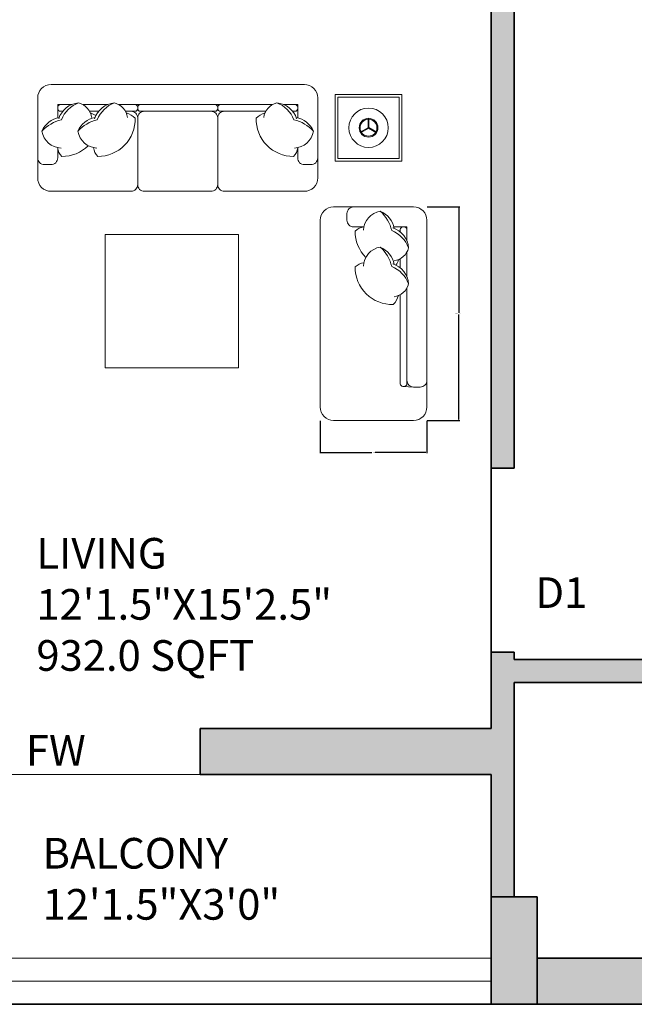
# Model space of a CAD drawing. Units: inches. Extents: x -9 to 505, y -680 to 48.
# Tile 4 of 17: x 235 to 356, y -680 to -487. Entities that reach past the tile are written whole.
import ezdxf

# ---------------------------------------------------------------- set-up
doc = ezdxf.new("R2010")
doc.units = ezdxf.units.IN
doc.header["$MEASUREMENT"] = 0
for name, color, linetype, lineweight in [('A-ANNO-DIMS', 2, 'Continuous', 18), ('A-ANNO-TEXT', 7, 'Continuous', 18), ('A-AREA-IDEN', 7, 'Continuous', 18), ('A-FLOR-HRAL', 4, 'Continuous', 18), ('A-FURN', 8, 'Continuous', 18), ('A-GLAZ', 4, 'Continuous', 18), ('A-WALL', 7, 'Continuous', 35), ('A-WALL-PATT', 251, 'Continuous', 13), ('S-CONC', 7, 'Continuous', 35), ('S-CONC-PATT', 18, 'Continuous', 13)]:
    doc.layers.add(name, color=color, linetype=linetype, lineweight=lineweight)
doc.styles.get("Standard").update_dxf_attribs({"font": 'arial.ttf'})
doc.dimstyles.get("Standard").update_dxf_attribs({"dimtxt": 0.18, "dimasz": 0.18, "dimexe": 0.18, "dimexo": 0.0625, "dimgap": 0.09, "dimtad": 0, "dimtih": 1, "dimtoh": 1, "dimdec": 0, "dimzin": 0, "dimdsep": 46, "dimlunit": 3, "dimtxsty": 'Standard', "dimcen": 0.09, "dimadec": 0, "dimazin": 0, "dimtfac": 1, "dimtdec": 0, "dimtofl": 0, "dimtmove": 0, "dimatfit": 3, "dimfxl": 1, "dimtolj": 1, "dimtzin": 0, "dimarcsym": 0})

# ---------------------------------------------------------------- blocks, each defined once
blk = doc.blocks.new('DAY BED1')
at = {"color": 0}
blk.add_line((0.3, 0.25), (0.225, 0.2549), dxfattribs=at)
blk.add_lwpolyline([(-0.3, 0, -0.414214), (-0.4, 0.1), (-0.4, 0.1, 0.317837), (-0.4, 0.1, -0.414214), (-0.4, 0.1), (-0.4, 0.1, 1.186185), (-0.4, 0.1, -0.414214), (-0.4, 0.1), (-0.4, 1.5, -0.414214), (-0.3, 1.6), (0.3, 1.6, -0.414214), (0.4, 1.5), (0.4, 0.1, -0.414214), (0.3, 0)], format="xyb", close=True, dxfattribs=at)
for points in [[(-0.0725, 1.45), (-0.15, 1.45, -0.414214), (-0.2, 1.5), (-0.2, 1.55, -0.414214), (-0.15, 1.6)], [(-0.0756, 1.4249, -0.356772), (0.0505, 1.5682, -0.249542), (0.1543, 1.4384, 9.61688)], [(0.0505, 1.5682, -0.14773), (0.1364, 1.422, -0.213343), (0.2624, 1.2931, -0.178662)], [(-0.0725, 1.4501, 0.165541), (-0.1386, 1.4192, 0.200231), (-0.0581, 1.2207, 0.121523)], [(0.1433, 1.4422, -0.306663), (0.2624, 1.2931, -0.30633), (0.1536, 1.1957, 0.872847)], [(0.25, 1.3448), (0.25, 1.45), (0.1517, 1.45, -0.414214)], [(0.2, 1.4118), (0.2, 1.43, -0.414214), (0.22, 1.45), (0.23, 1.45, -0.414214), (0.25, 1.43)], [(0.25, 1.43), (0.25, 1.3448, -0.414214)], [(-0.0756, 1.1556, -0.356772), (0.0505, 1.2988, -0.249542), (0.1543, 1.169, 9.61688)], [(0.0505, 1.2988, -0.14773), (0.1364, 1.1527, -0.213343), (0.2624, 1.0238, -0.178662)], [(0.25, 1.2616), (0.25, 1.0755, -0.414214)], [(-0.0725, 1.1808, 0.165541), (-0.1386, 1.1498, 0.425989), (0.1479, 0.869, 0.121523), (0.1873, 0.9357, -7.115464)], [(0.1678, 1.1631, 0.071865), (0.1873, 1.205, -7.115464)], [(0.2, 1.1425), (0.2, 1.2113, -0.414214)], [(0.1433, 1.1729, -0.306663), (0.2624, 1.0238, -0.30633), (0.1536, 0.9263, 0.872847)], [(0.25, 0.9923), (0.25, 0.2749, -0.414214), (0.23, 0.2549), (0.22, 0.2549, -0.414214), (0.2, 0.2749), (0.2, 0.9419, -0.414214)], [(0.25, 0.3775), (0.25, 0.3, 0.414214), (0.3, 0.25), (0.35, 0.25, 0.414214), (0.4, 0.3)]]:
    blk.add_lwpolyline(points, format="xyb", dxfattribs=at)
for points in [[(0.25, 1.0755), (0.25, 1.2616)], [(0.25, 0.3775), (0.25, 0.9923)]]:
    blk.add_lwpolyline(points, dxfattribs=at)
blk = doc.blocks.new('TABLE-COFFEE-SQUARE')
at = {"ltscale": 0.03}
blk.add_lwpolyline([(0, 0), (26.11, 0), (26.11, 26.11), (0, 26.11)], close=True, dxfattribs=at)
blk = doc.blocks.new('*D44')
at = {"layer": 'A-ANNO-DIMS', "color": 0, "lineweight": -2, "transparency": 16777216}
for p, q in [((315.22, -523.45), (321.6, -523.45)), ((321.42, -523.63), (321.42, -544.16)), ((321.42, -565.05), (321.42, -544.52)), ((315.22, -565.23), (321.6, -565.23))]:
    blk.add_line(p, q, dxfattribs=at)
at = {"layer": 'A-ANNO-DIMS', "color": 0, "transparency": 16777216}
for points in [[(321.39, -523.63), (321.45, -523.63), (321.42, -523.45)], [(321.39, -565.05), (321.45, -565.05), (321.42, -565.23)]]:
    blk.add_solid(points, dxfattribs=at)
at = {"layer": 'Defpoints', "color": 0, "transparency": 16777216}
for p in [(315.15, -523.45), (321.42, -523.45), (315.15, -565.23)]:
    blk.add_point(p, dxfattribs=at)
at = {"layer": 'A-ANNO-DIMS', "color": 0, "transparency": 16777216, "insert": (321.42, -544.34), "char_height": 0.18, "attachment_point": 5}
blk.add_mtext('\\A1;DAYBED 3\'-6"', dxfattribs=at)
blk = doc.blocks.new('*D45')
at = {"layer": 'A-ANNO-DIMS', "color": 0, "lineweight": -2, "transparency": 16777216}
for p, q in [((294.27, -565.29), (294.27, -571.67)), ((315.15, -565.29), (315.15, -571.67)), ((294.45, -571.49), (304.39, -571.49)), ((314.97, -571.49), (305.03, -571.49))]:
    blk.add_line(p, q, dxfattribs=at)
at = {"layer": 'A-ANNO-DIMS', "color": 0, "transparency": 16777216}
for points in [[(294.45, -571.46), (294.45, -571.52), (294.27, -571.49)], [(314.97, -571.46), (314.97, -571.52), (315.15, -571.49)]]:
    blk.add_solid(points, dxfattribs=at)
at = {"layer": 'Defpoints', "color": 0, "transparency": 16777216}
for p in [(294.27, -565.23), (315.15, -565.23), (315.15, -571.49)]:
    blk.add_point(p, dxfattribs=at)
at = {"layer": 'A-ANNO-DIMS', "color": 0, "transparency": 16777216, "insert": (304.71, -571.49), "char_height": 0.18, "attachment_point": 5}
blk.add_mtext('\\A1;1\'-9"', dxfattribs=at)

msp = doc.modelspace()

# ---------------------------------------------------------------- hatches: boundary and pattern name
at = {"layer": 'A-WALL-PATT'}
h = msp.add_hatch(color=256, dxfattribs=at)
h.dxf.hatch_style = 1
h.paths.add_polyline_path([(101.64, 11.5), (48.26, 11.5), (48.26, 2.5), (72.26, 2.5), (72.26, -21.25), (81.26, -21.25), (81.26, 2.5), (101.64, 2.5)])
h.paths.add_polyline_path([(36.26, 2.5), (27.26, 2.5), (27.26, -6.92), (36.26, -6.92)])
h.paths.add_polyline_path([(81.26, -57.25), (72.26, -57.25), (72.26, -75.5), (81.26, -75.5)])
h.paths.add_polyline_path([(162.76, 11.5), (137.64, 11.5), (137.64, 2.5), (162.76, 2.5)])
h.paths.add_polyline_path([(179.26, 2.5), (174.76, 2.5), (174.76, -75.5), (179.26, -75.5), (179.26, -54.5), (229.51, -54.5), (229.51, -45.5), (179.26, -45.5)])
h.paths.add_polyline_path([(382.26, -45.5), (332.26, -45.5), (332.26, 2.5), (327.76, 2.5), (327.76, -45.5), (277.51, -45.5), (277.51, -54.5), (327.76, -54.5), (327.76, -111.5), (332.26, -111.5), (332.26, -54.5), (382.26, -54.5)])
h.paths.add_polyline_path([(332.26, -128), (327.76, -128), (327.76, -207), (332.26, -207)])
h.paths.add_polyline_path([(124.76, -111.5), (36.26, -111.5), (36.26, -116), (120.26, -116), (120.26, -168.5), (179.26, -168.5), (179.26, -164), (124.76, -164)])
h.paths.add_polyline_path([(96.26, -164), (36.26, -164), (36.26, -152), (27.26, -152), (27.26, -208.88), (36.26, -208.88), (36.26, -168.5), (96.26, -168.5)])
h.paths.add_polyline_path([(36.26, -244.88), (27.26, -244.88), (27.26, -287), (36.26, -287)])
h.paths.add_polyline_path([(179.26, -204.5), (174.76, -204.5), (174.76, -287), (179.26, -287)])
h.paths.add_polyline_path([(257.26, -296), (248.26, -296), (248.26, -446), (269.26, -446), (269.26, -437), (257.26, -437)])
h.paths.add_polyline_path([(90.26, -296), (81.26, -296), (81.26, -348.67), (90.26, -348.67)])
h.paths.add_polyline_path([(90.26, -384.67), (81.26, -384.67), (81.26, -416), (90.26, -416)])
h.paths.add_polyline_path([(170.26, -452), (36.26, -452), (36.26, -456.5), (165.76, -456.5), (165.76, -504.5), (165.13, -504.5), (165.13, -509), (170.26, -509)])
h.paths.add_polyline_path([(141.76, -504.5), (36.26, -504.5), (36.26, -492.5), (27.26, -492.5), (27.26, -565.96), (36.26, -565.96), (36.26, -509), (141.76, -509)])
h.paths.add_polyline_path([(36.26, -601.96), (27.26, -601.96), (27.26, -658.5), (36.26, -658.5)])
h.paths.add_polyline_path([(170.26, -670.5), (170.26, -634.5), (222.76, -634.5), (222.76, -625.5), (165.76, -625.5), (165.76, -670.5), (36.26, -670.5), (36.26, -679.5), (170.26, -679.5)])
h.paths.add_polyline_path([(332.26, -616.5), (433.89, -616.5), (433.89, -612), (332.26, -612), (332.26, -610.56), (327.76, -610.56), (327.76, -625.5), (270.76, -625.5), (270.76, -634.5), (327.76, -634.5), (327.76, -658.5), (332.26, -658.5)])
h.paths.add_polyline_path([(459.76, -670.5), (336.76, -670.5), (336.76, -679.5), (459.76, -679.5)])
h.paths.add_polyline_path([(468.76, -545.74), (459.76, -545.74), (459.76, -612), (457.89, -612), (457.89, -616.5), (459.76, -616.5), (459.76, -658.5), (468.76, -658.5)])
h.paths.add_polyline_path([(332.26, -446), (327.76, -446), (327.76, -574.56), (332.26, -574.56)])
h.paths.add_polyline_path([(327.76, -437), (305.26, -437), (305.26, -446), (327.76, -446)])
h.paths.add_polyline_path([(459.76, -437), (348.76, -437), (348.76, -446), (459.76, -446)])
h.paths.add_polyline_path([(468.76, -458), (459.76, -458), (459.76, -509.74), (468.76, -509.74)])
h.paths.add_polyline_path([(468.76, -365), (459.76, -365), (459.76, -437), (468.76, -437)])
h.paths.add_polyline_path([(468.76, -299.6), (459.76, -299.6), (459.76, -344), (468.76, -344)])
h.paths.add_polyline_path([(468.76, -184.74), (459.76, -184.74), (459.76, -231), (401.26, -231), (401.26, -235.5), (459.76, -235.5), (459.76, -275.6), (468.76, -275.6)])
h.paths.add_polyline_path([(390.76, -356), (342.76, -356), (342.76, -365), (390.76, -365)])
h.paths.add_polyline_path([(459.76, -356), (405.76, -356), (405.76, -365), (459.76, -365)])
h.paths.add_polyline_path([(405.76, -296), (396.76, -296), (396.76, -356), (405.76, -356)])
h.paths.add_polyline_path([(336.76, -296), (327.76, -296), (327.76, -356), (336.76, -356)])
h.paths.add_polyline_path([(468.76, -9.5), (459.76, -9.5), (459.76, -45.5), (418.26, -45.5), (418.26, -54.5), (468.76, -54.5)])
h.paths.add_polyline_path([(468.76, -54.5), (459.76, -54.5), (459.76, -111.5), (468.76, -111.5)])
h.paths.add_polyline_path([(468.76, -128), (459.76, -128), (459.76, -148.74), (468.76, -148.74)])
at = {"layer": 'S-CONC-PATT'}
h = msp.add_hatch(color=256, dxfattribs=at)
h.dxf.hatch_style = 1
h.paths.add_polyline_path([(336.76, -658.5), (327.76, -658.5), (327.76, -679.5), (336.76, -679.5), (336.76, -670.5)])
h.paths.add_polyline_path([(468.76, -658.5), (459.76, -658.5), (459.76, -679.5), (468.76, -679.5)])
h.paths.add_polyline_path([(36.26, -658.5), (27.26, -658.5), (27.26, -679.5), (36.26, -679.5)])

# ---------------------------------------------------------------- linework, layer by layer
at = {"layer": 'A-FLOR-HRAL'}
for p, q in [((327.76, -670.5), (170.26, -670.5)), ((170.26, -670.5), (327.76, -670.5)), ((327.76, -679.5), (327.76, -670.5)), ((170.26, -675), (327.76, -675)), ((170.26, -679.5), (327.76, -679.5))]:
    msp.add_line(p, q, dxfattribs=at)
at = {"layer": 'A-FURN'}
for p, q in [((303.64, -507.96), (303.64, -506.12)), ((303.81, -507.96), (303.81, -506.12)), ((303.69, -507.89), (302.09, -508.81)), ((303.77, -508.03), (302.17, -508.95)), ((303.69, -508.03), (305.28, -508.95)), ((303.77, -507.89), (305.36, -508.81))]:
    msp.add_line(p, q, dxfattribs=at)
at = {"layer": 'A-FURN', "ltscale": 0.03}
msp.add_lwpolyline([(293.77, -517.79, -0.414214), (291.16, -520.4), (275.49, -520.4, -0.414214), (274.19, -519.09, -0.414214), (272.88, -520.4), (259.83, -520.4, -0.414214), (258.52, -519.09, -0.414214), (257.22, -520.4), (241.55, -520.4, -0.414214), (238.94, -517.79), (238.94, -502.12, -0.414214), (241.55, -499.51), (291.16, -499.51, -0.414214), (293.77, -502.12)], format="xyb", close=True, dxfattribs=at)
msp.add_lwpolyline([(310.25, -514.49), (297.2, -514.49), (297.2, -501.43), (310.25, -501.43)], close=True, dxfattribs=at)
at = {"layer": 'A-FURN'}
msp.add_lwpolyline([(297.72, -513.97), (309.73, -513.97), (309.73, -501.96), (297.72, -501.96)], close=True, dxfattribs=at)
for points in [[(239.77, -508.64, -0.14773), (243.59, -506.39, -0.213343), (246.95, -503.1, -0.178662)], [(245.6, -503.43), (242.86, -503.43), (242.86, -505.99, -0.414214)], [(243.85, -504.73), (243.38, -504.73, -0.414214), (242.86, -504.21), (242.86, -503.95, -0.414214), (243.38, -503.43)], [(243.06, -506.22, -0.306663), (246.95, -503.1, -0.30633), (249.5, -505.95, 0.872847)], [(243.38, -503.43), (245.6, -503.43, -0.414214)], [(246.8, -508.64, -0.14773), (250.62, -506.39, -0.213343), (253.98, -503.1, -0.178662)], [(247.77, -503.43), (252.63, -503.43, -0.414214)], [(250.88, -504.73), (249.09, -504.73, -0.414214)], [(250.09, -506.22, -0.306663), (253.98, -503.1, -0.30633), (256.53, -505.95, 0.872847)], [(254.81, -503.43), (258, -503.43, -0.414214), (258.52, -503.95), (258.52, -504.21, -0.414214), (258, -504.73), (256.12, -504.73, -0.414214)], [(257.22, -504.73, -0.414214), (258.52, -506.04), (258.52, -519.09, -0.414214)], [(259.83, -504.73, 0.414214), (258.52, -506.04)], [(272.88, -504.73, -0.414214), (274.19, -506.04)], [(284.94, -503.43), (274.71, -503.43, 0.414214), (274.19, -503.95), (274.19, -504.21, 0.414214), (274.71, -504.73), (283.62, -504.73, 0.414214)], [(275.49, -504.73, 0.414214), (274.19, -506.04), (274.19, -519.09, 0.414214)], [(289.65, -506.22, 0.306663), (285.76, -503.1, 0.30633), (283.21, -505.95, -0.872847)], [(292.94, -508.64, 0.14773), (289.12, -506.39, 0.213343), (285.76, -503.1, 0.178662)], [(289.33, -503.43), (287.11, -503.43, 0.414214)], [(288.86, -504.73), (289.33, -504.73, 0.414214), (289.85, -504.21), (289.85, -503.95, 0.414214), (289.33, -503.43)], [(243.51, -511.93, -0.356772), (239.77, -508.64, -0.249542), (243.16, -505.93, 9.61688)], [(250.54, -511.93, -0.356772), (246.8, -508.64, -0.249542), (250.19, -505.93, 9.61688)], [(250.35, -505.57, 0.071865), (249.25, -505.06, -7.115464)], [(249.89, -511.85, 0.165541), (250.69, -513.57, 0.425989), (258.02, -506.09, 0.121523), (256.28, -505.06, -7.115464)], [(289.86, -511.85, -0.165541), (289.05, -513.57, -0.425989), (281.72, -506.09, -0.121523), (283.46, -505.06, 7.115464)], [(289.2, -511.93, 0.356772), (292.94, -508.64, 0.249542), (289.55, -505.93, -9.61688)], [(242.86, -511.85), (242.86, -513.87, -0.414214), (241.55, -515.18), (240.24, -515.18, -0.414214), (238.94, -513.87)], [(242.85, -511.85, 0.165541), (243.66, -513.57, 0.200231), (248.84, -511.47, 0.121523)], [(293.77, -513.87, -0.414214), (292.46, -515.18), (291.16, -515.18, -0.414214), (289.85, -513.87), (289.85, -511.85)]]:
    msp.add_lwpolyline(points, format="xyb", dxfattribs=at)
for points in [[(252.63, -503.43), (247.77, -503.43)], [(284.94, -503.43), (254.81, -503.43)], [(289.85, -505.99), (289.85, -503.43), (287.11, -503.43)]]:
    msp.add_lwpolyline(points, dxfattribs=at)
msp.add_lwpolyline([(259.04, -503.43), (273.67, -503.43, -0.414214), (274.19, -503.95), (274.19, -504.21, -0.414214), (273.67, -504.73), (259.04, -504.73, -0.414214), (258.52, -504.21), (258.52, -503.95, -0.414214)], format="xyb", close=True, dxfattribs=at)
for radius in [3.85, 1.84, 1.65]:
    msp.add_circle((303.73, -507.96), radius, dxfattribs=at)
at = {"layer": 'A-GLAZ'}
msp.add_line((222.76, -634.5), (270.76, -634.5), dxfattribs=at)
at = {"layer": 'A-WALL'}
for p, q in [((327.76, -437), (327.76, -625.5)), ((332.26, -446), (332.26, -574.56)), ((327.76, -574.56), (332.26, -574.56)), ((332.26, -610.56), (327.76, -610.56)), ((332.26, -610.56), (332.26, -612)), ((332.26, -612), (433.89, -612)), ((332.26, -616.5), (433.89, -616.5)), ((332.26, -616.5), (332.26, -658.5)), ((270.76, -634.5), (270.76, -625.5)), ((270.76, -625.5), (327.76, -625.5)), ((270.76, -634.5), (327.76, -634.5)), ((327.76, -634.5), (327.76, -679.5)), ((336.76, -670.5), (459.76, -670.5)), ((27.26, -679.5), (468.76, -679.5))]:
    msp.add_line(p, q, dxfattribs=at)
at = {"layer": 'S-CONC'}
for p, q in [((336.76, -658.5), (327.76, -658.5)), ((336.76, -670.5), (336.76, -658.5)), ((336.76, -670.5), (336.76, -679.5))]:
    msp.add_line(p, q, dxfattribs=at)

# ---------------------------------------------------------------- block references
at = {"layer": 'A-FURN', "ltscale": 0.03, "xscale": 26.10992115726978, "yscale": 26.10992115726978, "zscale": 26.10992115726978}
msp.add_blockref('DAY BED1', (304.71, -565.23), dxfattribs=at)
at = {"layer": 'A-FURN'}
msp.add_blockref('TABLE-COFFEE-SQUARE', (252.16, -554.96), dxfattribs=at)

# ---------------------------------------------------------------- texts
at = {"layer": 'A-ANNO-TEXT', "insert": (336.39, -595.94), "char_height": 6, "attachment_point": 1}
msp.add_mtext('D1', dxfattribs=at)
at = {"layer": 'A-ANNO-TEXT', "insert": (236.64, -626.82), "char_height": 6, "attachment_point": 1}
msp.add_mtext_dynamic_manual_height_columns('FW', width=0.3247, gutter_width=1, heights=[0], dxfattribs=at)
at = {"layer": 'A-AREA-IDEN', "char_height": 6, "attachment_point": 1}
for s, insert in [('LIVING\\P12\'1.5"X15\'2.5"\\P932.0 SQFT', (238.68, -588.24)), ('BALCONY\\P12\'1.5"X3\'0"', (239.89, -646.94))]:
    msp.add_mtext(s, dxfattribs=dict(at, insert=insert))

# ---------------------------------------------------------------- dimensions: what is measured, and where the dimension line sits
at = {"layer": 'A-ANNO-DIMS'}
dim = msp.add_linear_dim(base=(321.42, -523.45), p1=(315.15, -565.23), p2=(315.15, -523.45), angle=90, text='DAYBED <>', dimstyle='Standard', override={"dimdec": 1, "dimlfac": 1, "dimrnd": 0, "dimzin": 1, "dimdsep": 46, "dimlunit": 4, "dimfrac": 2}, dxfattribs=at)
dim.commit()
dim.dimension.update_dxf_attribs({"geometry": '*D44', "text_midpoint": (321.42, -544.34)})
dim = msp.add_linear_dim(base=(315.15, -571.49), p1=(294.27, -565.23), p2=(315.15, -565.23), dimstyle='Standard', override={"dimdec": 1, "dimlfac": 1, "dimrnd": 0, "dimzin": 1, "dimdsep": 46, "dimlunit": 4, "dimfrac": 2}, dxfattribs=at)
dim.commit()
dim.dimension.update_dxf_attribs({"geometry": '*D45', "text_midpoint": (304.71, -571.49)})

doc.saveas('drawing.dxf')
